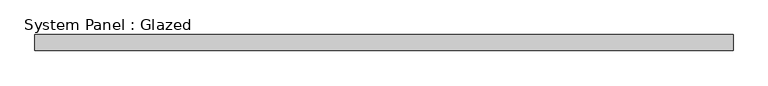
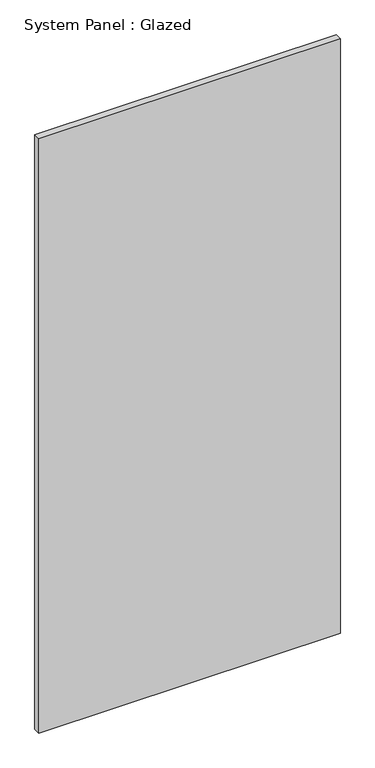
"""IFC4 building model written with IfcOpenShell, lengths in millimetres: plate geometry, System Panel : Glazed."""

from ifc_helpers import new_model, si_unit, origin, origin_with_axes, place, context, project, spatial, polyline, outline, extrude, source, transform, mapped, element, save


def system_panel_glazed_d43da186(model_context):
    return source(origin(), model_context, "Body", "SweptSolid", [
        extrude(outline(polyline([(552.4500001, 19.05), (-552.4500001, 19.05), (-552.4500001, 44.45), (552.4500001, 44.45), (552.4500001, 19.05)])), origin_with_axes(), (0.0, 0.0, 1.0), 2301.9640157),
    ])


if __name__ == "__main__":
    model = new_model("IFC4")
    model_context = context("Model", 3, world=origin())
    ifc_project = project(units=[si_unit("LENGTHUNIT", "METRE", prefix="MILLI")], contexts=[model_context])
    site = spatial("IfcSite", under=ifc_project)
    building = spatial("IfcBuilding", under=site)
    placement = place(None, origin())
    system_panel_glazed_shape = system_panel_glazed_d43da186(model_context)
    element("IfcPlate", 1, ObjectType="System Panel : Glazed", at=placement, inside=building, context=model_context, shape_type="MappedRepresentation", body=[
        mapped(system_panel_glazed_shape, transform((0.0, 0.0, 0.0), x_axis=(1.0, 0.0, 0.0), y_axis=(0.0, 1.0, 0.0), z_axis=(0.0, 0.0, 1.0))),
    ])
    save(model, "model.ifc")

# Revit data of these elements
# Type "System Panel : Glazed"
#   Construction Type Id = "GSP4R"
#   Analytic Construction = "1/8 in Pilkington single glazing"
#   Visual Light Transmittance = 0.9
#   Solar Heat Gain Coefficient = 0.86
#   Heat Transfer Coefficient (U) = 1.18115 BTU/(h·ft²·°F)
#   Define Thermal Properties by = 1
# Element 1 (IfcPlate, "System Panel : Glazed")
#   Materials on its faces: "Glass"
# Materials
#   "Glass": class "Glass", colour RGB 0 128 192, transparency 0.75, Description = "Soda Lime Glass", Cost = 0
